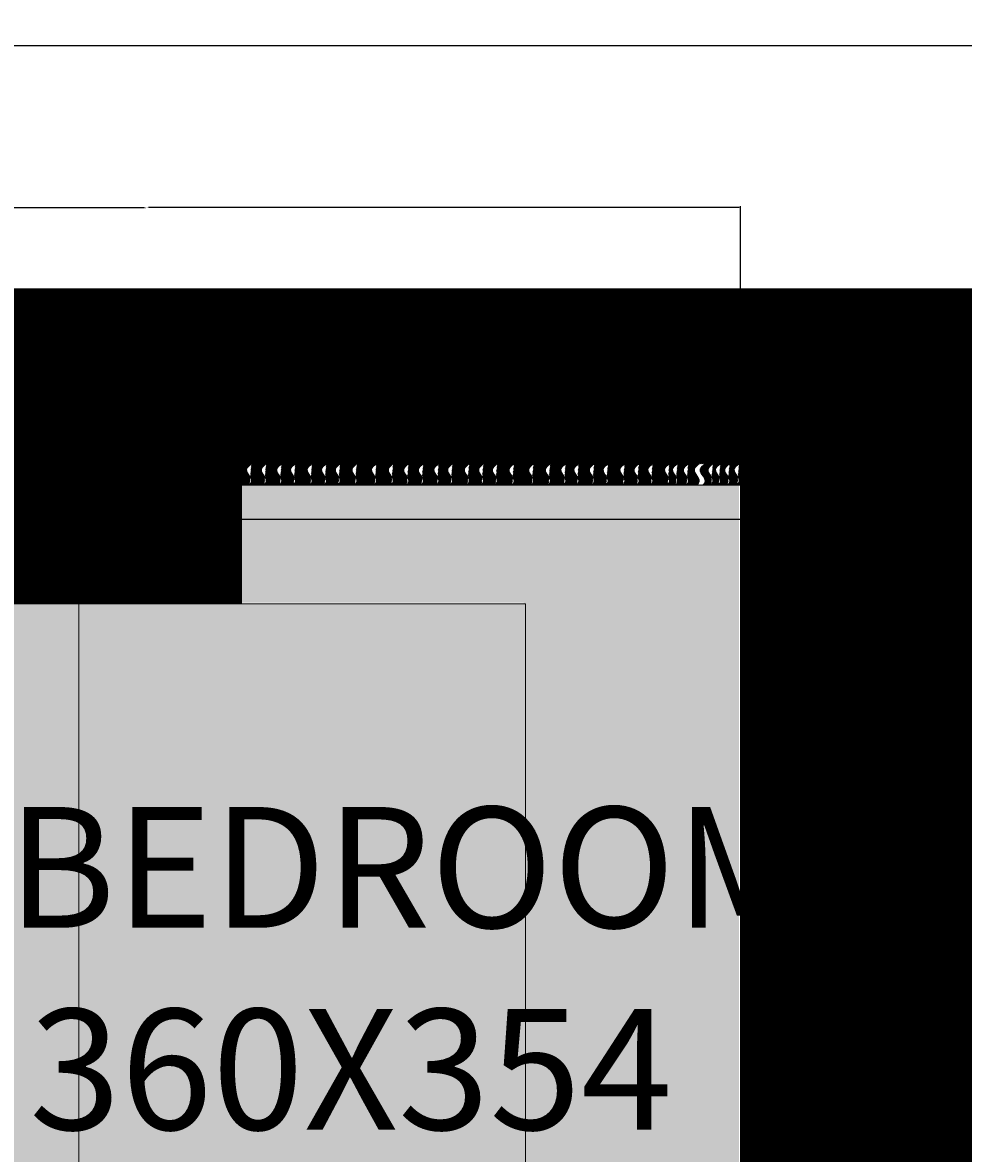
# Model space of a CAD drawing. Units: inches. Extents: x 192 to 1361, y -1362 to 367.
# Tile 8 of 23: x 361 to 495, y -616 to -454. Entities that reach past the tile are written whole.
import ezdxf

# ---------------------------------------------------------------- set-up
doc = ezdxf.new("R2010")
doc.units = ezdxf.units.IN
doc.header["$MEASUREMENT"] = 0
for name, color, linetype, lineweight in [('A-ANNO-DIMS', 2, 'Continuous', 18), ('A-AREA-IDEN', 7, 'Continuous', 18), ('A-FLOR', 8, 'Continuous', 18), ('furniture', 32, 'Continuous', 18)]:
    doc.layers.add(name, color=color, linetype=linetype, lineweight=lineweight)
doc.layers.add('A-FLOR-PATT', color=254, linetype='Continuous', lineweight=13, true_color=0xfeeab9)
doc.layers.add('A-FURN-PATT', color=254, linetype='Continuous', lineweight=13, true_color=0xfeeab9)
doc.styles.get("Standard").update_dxf_attribs({"font": 'arial.ttf'})
doc.dimstyles.get("Standard").update_dxf_attribs({"dimtxt": 0.18, "dimasz": 0.18, "dimexe": 0.18, "dimexo": 0.0625, "dimgap": 0.09, "dimtad": 0, "dimtih": 1, "dimtoh": 1, "dimzin": 0, "dimdsep": 46, "dimlunit": 3, "dimtxsty": 'Standard', "dimcen": 0.09, "dimadec": 0, "dimazin": 0, "dimtfac": 1, "dimtofl": 0, "dimtmove": 0, "dimatfit": 3, "dimfxl": 1, "dimtolj": 1, "dimtzin": 0, "dimarcsym": 0})

# ---------------------------------------------------------------- blocks, each defined once
blk = doc.blocks.new('CARPET')
at = {"layer": 'furniture'}
for p, q in [((-51.535, -98.109), (-51.535, -55.124)), ((-51.535, -55.124), (-41.267, -55.124)), ((51.553, -98.109), (-51.535, -98.109))]:
    blk.add_line(p, q, dxfattribs=at)
for points, knots in [([(-53.374, -55.995), (-53.215, -55.797), (-52.902, -55.407), (-52.343, -55.797), (-51.889, -56.079), (-51.645, -55.906), (-51.535, -55.827)], [0, 0, 0, 0, 0.653278, 1.290138, 1.740457, 2.114451, 2.114451, 2.114451, 2.114451]), ([(-53.374, -57.263), (-53.215, -57.065), (-52.902, -56.675), (-52.343, -57.065), (-51.889, -57.347), (-51.645, -57.174), (-51.535, -57.095)], [0, 0, 0, 0, 0.653278, 1.290138, 1.740457, 2.114451, 2.114451, 2.114451, 2.114451]), ([(-53.374, -58.593), (-53.215, -58.395), (-52.902, -58.005), (-52.343, -58.395), (-51.889, -58.678), (-51.645, -58.504), (-51.535, -58.426)], [0, 0, 0, 0, 0.653278, 1.290138, 1.740457, 2.114451, 2.114451, 2.114451, 2.114451]), ([(-53.374, -59.78), (-53.215, -59.582), (-52.902, -59.192), (-52.343, -59.582), (-51.889, -59.864), (-51.645, -59.691), (-51.535, -59.612)], [0, 0, 0, 0, 0.653278, 1.290138, 1.740457, 2.114451, 2.114451, 2.114451, 2.114451]), ([(-53.374, -61.218), (-53.215, -61.02), (-52.902, -60.63), (-52.343, -61.02), (-51.889, -61.302), (-51.645, -61.129), (-51.535, -61.051)], [0, 0, 0, 0, 0.653278, 1.290138, 1.740457, 2.114451, 2.114451, 2.114451, 2.114451]), ([(-53.374, -62.444), (-53.215, -62.247), (-52.902, -61.857), (-52.343, -62.247), (-51.889, -62.529), (-51.645, -62.355), (-51.535, -62.277)], [0, 0, 0, 0, 0.653278, 1.290138, 1.740457, 2.114451, 2.114451, 2.114451, 2.114451]), ([(-53.374, -63.631), (-53.215, -63.433), (-52.902, -63.043), (-52.343, -63.433), (-51.889, -63.715), (-51.645, -63.542), (-51.535, -63.463)], [0, 0, 0, 0, 0.653278, 1.290138, 1.740457, 2.114451, 2.114451, 2.114451, 2.114451]), ([(-53.374, -65.069), (-53.215, -64.872), (-52.902, -64.481), (-52.343, -64.871), (-51.889, -65.154), (-51.645, -64.98), (-51.535, -64.902)], [0, 0, 0, 0, 0.653278, 1.290138, 1.740457, 2.114451, 2.114451, 2.114451, 2.114451]), ([(-53.374, -66.759), (-53.215, -66.561), (-52.902, -66.171), (-52.343, -66.561), (-51.889, -66.844), (-51.645, -66.67), (-51.535, -66.592)], [0, 0, 0, 0, 0.653278, 1.290138, 1.740457, 2.114451, 2.114451, 2.114451, 2.114451]), ([(-53.374, -68.197), (-53.215, -68), (-52.902, -67.61), (-52.343, -68), (-51.889, -68.282), (-51.645, -68.109), (-51.535, -68.03)], [0, 0, 0, 0, 0.653278, 1.290138, 1.740457, 2.114451, 2.114451, 2.114451, 2.114451]), ([(-53.374, -69.528), (-53.215, -69.33), (-52.902, -68.94), (-52.343, -69.33), (-51.889, -69.612), (-51.645, -69.439), (-51.535, -69.36)], [0, 0, 0, 0, 0.653278, 1.290138, 1.740457, 2.114451, 2.114451, 2.114451, 2.114451]), ([(-53.374, -70.794), (-53.215, -70.596), (-52.902, -70.206), (-52.343, -70.596), (-51.889, -70.878), (-51.645, -70.705), (-51.535, -70.626)], [0, 0, 0, 0, 0.653278, 1.290138, 1.740457, 2.114451, 2.114451, 2.114451, 2.114451]), ([(-53.374, -72.124), (-53.215, -71.927), (-52.902, -71.536), (-52.343, -71.927), (-51.889, -72.209), (-51.645, -72.035), (-51.535, -71.957)], [0, 0, 0, 0, 0.653278, 1.290138, 1.740457, 2.114451, 2.114451, 2.114451, 2.114451]), ([(-53.374, -73.311), (-53.215, -73.113), (-52.902, -72.723), (-52.343, -73.113), (-51.889, -73.395), (-51.645, -73.222), (-51.535, -73.143)], [0, 0, 0, 0, 0.653278, 1.290138, 1.740457, 2.114451, 2.114451, 2.114451, 2.114451]), ([(-53.374, -74.749), (-53.215, -74.551), (-52.902, -74.161), (-52.343, -74.551), (-51.889, -74.833), (-51.645, -74.66), (-51.535, -74.582)], [0, 0, 0, 0, 0.653278, 1.290138, 1.740457, 2.114451, 2.114451, 2.114451, 2.114451]), ([(-53.374, -75.975), (-53.215, -75.778), (-52.902, -75.388), (-52.343, -75.778), (-51.889, -76.06), (-51.645, -75.887), (-51.535, -75.808)], [0, 0, 0, 0, 0.653278, 1.290138, 1.740457, 2.114451, 2.114451, 2.114451, 2.114451]), ([(-53.374, -77.162), (-53.215, -76.964), (-52.902, -76.574), (-52.343, -76.964), (-51.889, -77.246), (-51.645, -77.073), (-51.535, -76.995)], [0, 0, 0, 0, 0.653278, 1.290138, 1.740457, 2.114451, 2.114451, 2.114451, 2.114451]), ([(-53.374, -78.6), (-53.215, -78.403), (-52.902, -78.012), (-52.343, -78.403), (-51.889, -78.685), (-51.645, -78.511), (-51.535, -78.433)], [0, 0, 0, 0, 0.653278, 1.290138, 1.740457, 2.114451, 2.114451, 2.114451, 2.114451]), ([(-53.374, -80.29), (-53.215, -80.093), (-52.902, -79.702), (-52.343, -80.093), (-51.889, -80.375), (-51.645, -80.201), (-51.535, -80.123)], [0, 0, 0, 0, 0.653278, 1.290138, 1.740457, 2.114451, 2.114451, 2.114451, 2.114451]), ([(-53.374, -81.728), (-53.215, -81.531), (-52.902, -81.141), (-52.343, -81.531), (-51.889, -81.813), (-51.645, -81.64), (-51.535, -81.561)], [0, 0, 0, 0, 0.653278, 1.290138, 1.740457, 2.114451, 2.114451, 2.114451, 2.114451]), ([(-53.374, -83.059), (-53.215, -82.861), (-52.902, -82.471), (-52.343, -82.861), (-51.889, -83.143), (-51.645, -82.97), (-51.535, -82.891)], [0, 0, 0, 0, 0.653278, 1.290138, 1.740457, 2.114451, 2.114451, 2.114451, 2.114451]), ([(-53.374, -84.183), (-53.215, -83.985), (-52.902, -83.595), (-52.343, -83.985), (-51.889, -84.267), (-51.645, -84.094), (-51.535, -84.015)], [0, 0, 0, 0, 0.653278, 1.290138, 1.740457, 2.114451, 2.114451, 2.114451, 2.114451]), ([(-53.374, -85.513), (-53.215, -85.316), (-52.902, -84.926), (-52.343, -85.316), (-51.889, -85.598), (-51.645, -85.424), (-51.535, -85.346)], [0, 0, 0, 0, 0.653278, 1.290138, 1.740457, 2.114451, 2.114451, 2.114451, 2.114451]), ([(-53.374, -86.7), (-53.215, -86.502), (-52.902, -86.112), (-52.343, -86.502), (-51.889, -86.784), (-51.645, -86.611), (-51.535, -86.532)], [0, 0, 0, 0, 0.653278, 1.290138, 1.740457, 2.114451, 2.114451, 2.114451, 2.114451]), ([(-53.374, -88.138), (-53.215, -87.941), (-52.902, -87.55), (-52.343, -87.94), (-51.889, -88.223), (-51.645, -88.049), (-51.535, -87.971)], [0, 0, 0, 0, 0.653278, 1.290138, 1.740457, 2.114451, 2.114451, 2.114451, 2.114451]), ([(-53.374, -89.364), (-53.215, -89.167), (-52.902, -88.777), (-52.343, -89.167), (-51.889, -89.449), (-51.645, -89.276), (-51.535, -89.197)], [0, 0, 0, 0, 0.653278, 1.290138, 1.740457, 2.114451, 2.114451, 2.114451, 2.114451]), ([(-53.374, -90.551), (-53.215, -90.353), (-52.902, -89.963), (-52.343, -90.353), (-51.889, -90.635), (-51.645, -90.462), (-51.535, -90.384)], [0, 0, 0, 0, 0.653278, 1.290138, 1.740457, 2.114451, 2.114451, 2.114451, 2.114451]), ([(-53.374, -91.989), (-53.215, -91.792), (-52.902, -91.402), (-52.343, -91.792), (-51.889, -92.074), (-51.645, -91.9), (-51.535, -91.822)], [0, 0, 0, 0, 0.653278, 1.290138, 1.740457, 2.114451, 2.114451, 2.114451, 2.114451]), ([(-53.374, -92.689), (-53.216, -92.483), (-52.904, -92.076), (-52.346, -92.494), (-51.889, -92.773), (-51.645, -92.6), (-51.535, -92.522)], [0, 0, 0, 0, 0.663904, 1.307406, 1.757725, 2.131719, 2.131719, 2.131719, 2.131719]), ([(-53.374, -93.614), (-53.215, -93.416), (-52.902, -93.026), (-52.343, -93.416), (-51.889, -93.698), (-51.645, -93.525), (-51.535, -93.446)], [0, 0, 0, 0, 0.653278, 1.290138, 1.740457, 2.114451, 2.114451, 2.114451, 2.114451]), ([(-53.374, -94.548), (-53.215, -94.351), (-52.902, -93.96), (-52.343, -94.35), (-51.889, -94.633), (-51.645, -94.459), (-51.535, -94.381)], [0, 0, 0, 0, 0.653278, 1.290138, 1.740457, 2.114451, 2.114451, 2.114451, 2.114451]), ([(-53.374, -95.052), (-53.215, -94.854), (-52.902, -94.464), (-52.343, -94.854), (-51.889, -95.136), (-51.645, -94.963), (-51.535, -94.885)], [0, 0, 0, 0, 0.653278, 1.290138, 1.740457, 2.114451, 2.114451, 2.114451, 2.114451]), ([(-53.374, -95.735), (-53.215, -95.537), (-52.902, -95.147), (-52.343, -95.537), (-51.889, -95.819), (-51.645, -95.646), (-51.535, -95.567)], [0, 0, 0, 0, 0.653278, 1.290138, 1.740457, 2.114451, 2.114451, 2.114451, 2.114451]), ([(-53.374, -96.382), (-53.215, -96.185), (-52.902, -95.795), (-52.343, -96.185), (-51.889, -96.467), (-51.645, -96.294), (-51.535, -96.215)], [0, 0, 0, 0, 0.653278, 1.290138, 1.740457, 2.114451, 2.114451, 2.114451, 2.114451]), ([(-53.374, -97.173), (-53.215, -96.975), (-52.902, -96.585), (-52.343, -96.975), (-51.889, -97.257), (-51.645, -97.084), (-51.535, -97.006)], [0, 0, 0, 0, 0.653278, 1.290138, 1.740457, 2.114451, 2.114451, 2.114451, 2.114451]), ([(-53.374, -97.991), (-53.215, -97.793), (-52.902, -97.403), (-52.343, -97.793), (-51.889, -98.075), (-51.645, -97.902), (-51.535, -97.824)], [0, 0, 0, 0, 0.653278, 1.290138, 1.740457, 2.114451, 2.114451, 2.114451, 2.114451])]:
    blk.add_open_spline(points, degree=3, knots=knots, dxfattribs=at)
blk = doc.blocks.new('A$C58D270C6')
at = {"layer": 'furniture'}
blk.add_line((42.078, 108), (42.078, 36), dxfattribs=at)
blk.add_lwpolyline([(0, 108), (77.905, 108), (77.905, 36), (0, 36)], close=True, dxfattribs=at)
at = {"layer": 'furniture', "xscale": 0.9312884925094044, "yscale": 0.9312884925094044, "zscale": 0.9312884925094044, "rotation": 90}
blk.add_blockref('CARPET', (3.79, 74.474), dxfattribs=at)
blk = doc.blocks.new('*D23')
at = {"layer": 'A-ANNO-DIMS', "color": 0, "lineweight": -2, "transparency": 16777216}
for p, q in [((463.14, -508.44), (491.09, -508.44)), ((490.91, -508.62), (490.91, -601.06)), ((490.91, -693.87), (490.91, -601.42)), ((463.14, -694.05), (491.09, -694.05))]:
    blk.add_line(p, q, dxfattribs=at)
at = {"layer": 'A-ANNO-DIMS', "color": 0, "transparency": 16777216}
for points in [[(490.88, -508.62), (490.94, -508.62), (490.91, -508.44)], [(490.88, -693.87), (490.94, -693.87), (490.91, -694.05)]]:
    blk.add_solid(points, dxfattribs=at)
at = {"layer": 'Defpoints', "color": 0, "transparency": 16777216}
for p in [(463.07, -508.44), (463.07, -694.05), (490.91, -694.05)]:
    blk.add_point(p, dxfattribs=at)
at = {"layer": 'A-ANNO-DIMS', "color": 0, "transparency": 16777216, "insert": (490.91, -601.24), "char_height": 0.18, "attachment_point": 5}
blk.add_mtext('\\A1;BED 186', dxfattribs=at)
blk = doc.blocks.new('*D24')
at = {"layer": 'A-ANNO-DIMS', "color": 0, "lineweight": -2, "transparency": 16777216}
for p, q in [((293.48, -508.38), (293.48, -480.42)), ((293.66, -480.6), (378, -480.6)), ((462.89, -480.6), (378.56, -480.6)), ((463.07, -508.38), (463.07, -480.42))]:
    blk.add_line(p, q, dxfattribs=at)
at = {"layer": 'A-ANNO-DIMS', "color": 0, "transparency": 16777216}
for points in [[(293.66, -480.57), (293.66, -480.63), (293.48, -480.6)], [(462.89, -480.57), (462.89, -480.63), (463.07, -480.6)]]:
    blk.add_solid(points, dxfattribs=at)
at = {"layer": 'Defpoints', "color": 0, "transparency": 16777216}
for p in [(463.07, -480.6), (293.48, -508.44), (463.07, -508.44)]:
    blk.add_point(p, dxfattribs=at)
at = {"layer": 'A-ANNO-DIMS', "color": 0, "transparency": 16777216, "insert": (378.28, -480.6), "char_height": 0.18, "attachment_point": 5}
blk.add_mtext('\\A1;170', dxfattribs=at)
blk = doc.blocks.new('*D48')
at = {"layer": 'A-ANNO-DIMS', "color": 0, "lineweight": -2, "transparency": 16777216}
for p, q in [((325.63, 258.53), (192.16, 258.53)), ((192.34, 258.35), (192.34, -429.22)), ((192.34, -1117.14), (192.34, -429.58)), ((395.21, -1117.32), (192.16, -1117.32))]:
    blk.add_line(p, q, dxfattribs=at)
at = {"layer": 'A-ANNO-DIMS', "color": 0, "transparency": 16777216}
for points in [[(192.31, 258.35), (192.37, 258.35), (192.34, 258.53)], [(192.31, -1117.14), (192.37, -1117.14), (192.34, -1117.32)]]:
    blk.add_solid(points, dxfattribs=at)
at = {"layer": 'Defpoints', "color": 0, "transparency": 16777216}
for p in [(325.7, 258.53), (192.34, -1117.32), (395.28, -1117.32)]:
    blk.add_point(p, dxfattribs=at)
at = {"layer": 'A-ANNO-DIMS', "color": 0, "transparency": 16777216, "insert": (192.34, -429.4), "char_height": 0.18, "attachment_point": 5}
blk.add_mtext('\\A1;1375.9', dxfattribs=at)
blk = doc.blocks.new('*D69')
at = {"layer": 'A-ANNO-DIMS', "color": 0, "lineweight": -2, "transparency": 16777216}
for p, q in [((981.75, -457.5), (192.16, -457.5)), ((192.34, -457.68), (192.34, -491.13)), ((192.34, -524.95), (192.34, -491.5)), ((980.52, -525.13), (192.16, -525.13))]:
    blk.add_line(p, q, dxfattribs=at)
at = {"layer": 'A-ANNO-DIMS', "color": 0, "transparency": 16777216}
for points in [[(192.31, -457.68), (192.37, -457.68), (192.34, -457.5)], [(192.31, -524.95), (192.37, -524.95), (192.34, -525.13)]]:
    blk.add_solid(points, dxfattribs=at)
at = {"layer": 'Defpoints', "color": 0, "transparency": 16777216}
for p in [(981.81, -457.5), (192.34, -525.13), (980.58, -525.13)]:
    blk.add_point(p, dxfattribs=at)
at = {"layer": 'A-ANNO-DIMS', "color": 0, "transparency": 16777216, "insert": (192.34, -491.31), "char_height": 0.18, "attachment_point": 5}
blk.add_mtext('\\A1;67.63', dxfattribs=at)

msp = doc.modelspace()

# ---------------------------------------------------------------- hatches: boundary and pattern name
at = {"layer": 'A-FLOR-PATT'}
h = msp.add_hatch(dxfattribs=at)
h.set_pattern_fill('ANSI31', color=256)
edge = h.paths.add_edge_path()
edge.add_line((513.1511, -492.1899), (327.1032, -492.1899))
edge.add_line((327.1032, -492.1899), (327.1032, -508.439))
edge.add_line((327.1032, -508.439), (326.9465, -508.439))
edge.add_line((326.9465, -508.439), (326.6697, -537.1419))
edge.add_line((326.6697, -537.1419), (391.8439, -537.1419))
edge.add_line((391.8439, -537.1419), (391.8439, -520.2026))
edge.add_line((391.8439, -520.2026), (393.0084, -520.2026))
edge.add_spline(control_points=[(393.2858, -517.1545), (392.9584, -517.4172), (392.3119, -517.936), (392.9583, -518.8629), (393.4257, -519.6151), (393.1386, -520.0192), (393.0084, -520.2026)], knot_values=[0, 0, 0, 0, 0.65327829, 1.2901376, 1.74045698, 2.11445126, 2.11445126, 2.11445126, 2.11445126], degree=3, periodic=0)
edge.add_line((393.0084, -520.2026), (395.1098, -520.2026))
edge.add_spline(control_points=[(395.3872, -517.1545), (395.0598, -517.4172), (394.4133, -517.936), (395.0598, -518.8629), (395.5272, -519.6151), (395.2401, -520.0192), (395.1098, -520.2026)], knot_values=[0, 0, 0, 0, 0.65327829, 1.2901376, 1.74045698, 2.11445126, 2.11445126, 2.11445126, 2.11445126], degree=3, periodic=0)
edge.add_line((395.1098, -520.2026), (397.3144, -520.2026))
edge.add_spline(control_points=[(397.5918, -517.1545), (397.2644, -517.4172), (396.6179, -517.936), (397.2643, -518.8629), (397.7317, -519.6151), (397.4446, -520.0192), (397.3144, -520.2026)], knot_values=[0, 0, 0, 0, 0.65327829, 1.2901376, 1.74045698, 2.11445126, 2.11445126, 2.11445126, 2.11445126], degree=3, periodic=0)
edge.add_line((397.3144, -520.2026), (399.2806, -520.2026))
edge.add_spline(control_points=[(399.558, -517.1545), (399.2307, -517.4172), (398.5841, -517.936), (399.2306, -518.8629), (399.698, -519.6151), (399.4109, -520.0192), (399.2806, -520.2026)], knot_values=[0, 0, 0, 0, 0.65327829, 1.2901376, 1.74045698, 2.11445126, 2.11445126, 2.11445126, 2.11445126], degree=3, periodic=0)
edge.add_line((399.2806, -520.2026), (401.664, -520.2026))
edge.add_spline(control_points=[(401.9414, -517.1545), (401.614, -517.4172), (400.9675, -517.936), (401.6139, -518.8629), (402.0814, -519.6151), (401.7943, -520.0192), (401.664, -520.2026)], knot_values=[0, 0, 0, 0, 0.65327829, 1.2901376, 1.74045698, 2.11445126, 2.11445126, 2.11445126, 2.11445126], degree=3, periodic=0)
edge.add_line((401.664, -520.2026), (403.6961, -520.2026))
edge.add_spline(control_points=[(403.9735, -517.1545), (403.6461, -517.4172), (402.9996, -517.936), (403.6461, -518.8629), (404.1135, -519.6151), (403.8264, -520.0192), (403.6961, -520.2026)], knot_values=[0, 0, 0, 0, 0.65327829, 1.2901376, 1.74045698, 2.11445126, 2.11445126, 2.11445126, 2.11445126], degree=3, periodic=0)
edge.add_line((403.6961, -520.2026), (405.6624, -520.2026))
edge.add_spline(control_points=[(405.9398, -517.1545), (405.6124, -517.4172), (404.9659, -517.936), (405.6123, -518.8629), (406.0797, -519.6151), (405.7926, -520.0192), (405.6624, -520.2026)], knot_values=[0, 0, 0, 0, 0.65327829, 1.2901376, 1.74045698, 2.11445126, 2.11445126, 2.11445126, 2.11445126], degree=3, periodic=0)
edge.add_line((405.6624, -520.2026), (408.0457, -520.2026))
edge.add_spline(control_points=[(408.3231, -517.1545), (407.9958, -517.4172), (407.3493, -517.936), (407.9957, -518.8629), (408.4631, -519.6151), (408.176, -520.0192), (408.0457, -520.2026)], knot_values=[0, 0, 0, 0, 0.65327829, 1.2901376, 1.74045698, 2.11445126, 2.11445126, 2.11445126, 2.11445126], degree=3, periodic=0)
edge.add_line((408.0457, -520.2026), (410.8462, -520.2026))
edge.add_spline(control_points=[(411.1236, -517.1545), (410.7962, -517.4172), (410.1497, -517.936), (410.7961, -518.8629), (411.2635, -519.6151), (410.9764, -520.0192), (410.8462, -520.2026)], knot_values=[0, 0, 0, 0, 0.65327829, 1.2901376, 1.74045698, 2.11445126, 2.11445126, 2.11445126, 2.11445126], degree=3, periodic=0)
edge.add_line((410.8462, -520.2026), (413.2295, -520.2026))
edge.add_spline(control_points=[(413.5069, -517.1545), (413.1795, -517.4172), (412.533, -517.936), (413.1794, -518.8629), (413.6468, -519.6151), (413.3597, -520.0192), (413.2295, -520.2026)], knot_values=[0, 0, 0, 0, 0.65327829, 1.2901376, 1.74045698, 2.11445126, 2.11445126, 2.11445126, 2.11445126], degree=3, periodic=0)
edge.add_line((413.2295, -520.2026), (415.434, -520.2026))
edge.add_spline(control_points=[(415.7114, -517.1545), (415.3841, -517.4172), (414.7376, -517.936), (415.384, -518.8629), (415.8514, -519.6151), (415.5643, -520.0192), (415.434, -520.2026)], knot_values=[0, 0, 0, 0, 0.65327829, 1.2901376, 1.74045698, 2.11445126, 2.11445126, 2.11445126, 2.11445126], degree=3, periodic=0)
edge.add_line((415.434, -520.2026), (417.5321, -520.2026))
edge.add_spline(control_points=[(417.8095, -517.1545), (417.4821, -517.4172), (416.8356, -517.936), (417.482, -518.8629), (417.9494, -519.6151), (417.6623, -520.0192), (417.5321, -520.2026)], knot_values=[0, 0, 0, 0, 0.65327829, 1.2901376, 1.74045698, 2.11445126, 2.11445126, 2.11445126, 2.11445126], degree=3, periodic=0)
edge.add_line((417.5321, -520.2026), (419.7366, -520.2026))
edge.add_spline(control_points=[(420.014, -517.1545), (419.6867, -517.4172), (419.0401, -517.936), (419.6866, -518.8629), (420.154, -519.6151), (419.8669, -520.0192), (419.7366, -520.2026)], knot_values=[0, 0, 0, 0, 0.65327829, 1.2901376, 1.74045698, 2.11445126, 2.11445126, 2.11445126, 2.11445126], degree=3, periodic=0)
edge.add_line((419.7366, -520.2026), (421.7029, -520.2026))
edge.add_spline(control_points=[(421.9803, -517.1545), (421.6529, -517.4172), (421.0064, -517.936), (421.6528, -518.8629), (422.1202, -519.6151), (421.8331, -520.0192), (421.7029, -520.2026)], knot_values=[0, 0, 0, 0, 0.65327829, 1.2901376, 1.74045698, 2.11445126, 2.11445126, 2.11445126, 2.11445126], degree=3, periodic=0)
edge.add_line((421.7029, -520.2026), (424.0863, -520.2026))
edge.add_spline(control_points=[(424.3637, -517.1545), (424.0363, -517.4172), (423.3898, -517.936), (424.0362, -518.8629), (424.5036, -519.6151), (424.2165, -520.0192), (424.0863, -520.2026)], knot_values=[0, 0, 0, 0, 0.65327829, 1.2901376, 1.74045698, 2.11445126, 2.11445126, 2.11445126, 2.11445126], degree=3, periodic=0)
edge.add_line((424.0863, -520.2026), (426.1184, -520.2026))
edge.add_spline(control_points=[(426.3958, -517.1545), (426.0684, -517.4172), (425.4219, -517.936), (426.0683, -518.8629), (426.5357, -519.6151), (426.2486, -520.0192), (426.1184, -520.2026)], knot_values=[0, 0, 0, 0, 0.65327829, 1.2901376, 1.74045698, 2.11445126, 2.11445126, 2.11445126, 2.11445126], degree=3, periodic=0)
edge.add_line((426.1184, -520.2026), (428.0846, -520.2026))
edge.add_spline(control_points=[(428.362, -517.1545), (428.0346, -517.4172), (427.3881, -517.936), (428.0346, -518.8629), (428.502, -519.6151), (428.2149, -520.0192), (428.0846, -520.2026)], knot_values=[0, 0, 0, 0, 0.65327829, 1.2901376, 1.74045698, 2.11445126, 2.11445126, 2.11445126, 2.11445126], degree=3, periodic=0)
edge.add_line((428.0846, -520.2026), (430.468, -520.2026))
edge.add_spline(control_points=[(430.7454, -517.1545), (430.418, -517.4172), (429.7715, -517.936), (430.4179, -518.8629), (430.8853, -519.6151), (430.5983, -520.0192), (430.468, -520.2026)], knot_values=[0, 0, 0, 0, 0.65327829, 1.2901376, 1.74045698, 2.11445126, 2.11445126, 2.11445126, 2.11445126], degree=3, periodic=0)
edge.add_line((430.468, -520.2026), (433.2684, -520.2026))
edge.add_spline(control_points=[(433.5458, -517.1545), (433.2184, -517.4172), (432.5719, -517.936), (433.2184, -518.8629), (433.6858, -519.6151), (433.3987, -520.0192), (433.2684, -520.2026)], knot_values=[0, 0, 0, 0, 0.65327829, 1.2901376, 1.74045698, 2.11445126, 2.11445126, 2.11445126, 2.11445126], degree=3, periodic=0)
edge.add_line((433.2684, -520.2026), (435.6517, -520.2026))
edge.add_spline(control_points=[(435.9291, -517.1545), (435.6017, -517.4172), (434.9552, -517.936), (435.6017, -518.8629), (436.0691, -519.6151), (435.782, -520.0192), (435.6517, -520.2026)], knot_values=[0, 0, 0, 0, 0.65327829, 1.2901376, 1.74045698, 2.11445126, 2.11445126, 2.11445126, 2.11445126], degree=3, periodic=0)
edge.add_line((435.6517, -520.2026), (437.8563, -520.2026))
edge.add_spline(control_points=[(438.1337, -517.1545), (437.8063, -517.4172), (437.1598, -517.936), (437.8062, -518.8629), (438.2736, -519.6151), (437.9865, -520.0192), (437.8563, -520.2026)], knot_values=[0, 0, 0, 0, 0.65327829, 1.2901376, 1.74045698, 2.11445126, 2.11445126, 2.11445126, 2.11445126], degree=3, periodic=0)
edge.add_line((437.8563, -520.2026), (439.7189, -520.2026))
edge.add_spline(control_points=[(439.9963, -517.1545), (439.669, -517.4172), (439.0225, -517.936), (439.6689, -518.8629), (440.1363, -519.6151), (439.8492, -520.0192), (439.7189, -520.2026)], knot_values=[0, 0, 0, 0, 0.65327829, 1.2901376, 1.74045698, 2.11445126, 2.11445126, 2.11445126, 2.11445126], degree=3, periodic=0)
edge.add_line((439.7189, -520.2026), (441.9235, -520.2026))
edge.add_spline(control_points=[(442.2009, -517.1545), (441.8735, -517.4172), (441.227, -517.936), (441.8735, -518.8629), (442.3409, -519.6151), (442.0538, -520.0192), (441.9235, -520.2026)], knot_values=[0, 0, 0, 0, 0.65327829, 1.2901376, 1.74045698, 2.11445126, 2.11445126, 2.11445126, 2.11445126], degree=3, periodic=0)
edge.add_line((441.9235, -520.2026), (443.8898, -520.2026))
edge.add_spline(control_points=[(444.1672, -517.1545), (443.8398, -517.4172), (443.1933, -517.936), (443.8397, -518.8629), (444.3071, -519.6151), (444.02, -520.0192), (443.8898, -520.2026)], knot_values=[0, 0, 0, 0, 0.65327829, 1.2901376, 1.74045698, 2.11445126, 2.11445126, 2.11445126, 2.11445126], degree=3, periodic=0)
edge.add_line((443.8898, -520.2026), (446.2731, -520.2026))
edge.add_spline(control_points=[(446.5505, -517.1545), (446.2232, -517.4172), (445.5767, -517.936), (446.2231, -518.8629), (446.6905, -519.6151), (446.4034, -520.0192), (446.2731, -520.2026)], knot_values=[0, 0, 0, 0, 0.65327829, 1.2901376, 1.74045698, 2.11445126, 2.11445126, 2.11445126, 2.11445126], degree=3, periodic=0)
edge.add_line((446.2731, -520.2026), (448.3052, -520.2026))
edge.add_spline(control_points=[(448.5826, -517.1545), (448.2553, -517.4172), (447.6088, -517.936), (448.2552, -518.8629), (448.7226, -519.6151), (448.4355, -520.0192), (448.3052, -520.2026)], knot_values=[0, 0, 0, 0, 0.65327829, 1.2901376, 1.74045698, 2.11445126, 2.11445126, 2.11445126, 2.11445126], degree=3, periodic=0)
edge.add_line((448.3052, -520.2026), (450.2715, -520.2026))
edge.add_spline(control_points=[(450.5489, -517.1545), (450.2215, -517.4172), (449.575, -517.936), (450.2214, -518.8629), (450.6888, -519.6151), (450.4018, -520.0192), (450.2715, -520.2026)], knot_values=[0, 0, 0, 0, 0.65327829, 1.2901376, 1.74045698, 2.11445126, 2.11445126, 2.11445126, 2.11445126], degree=3, periodic=0)
edge.add_line((450.2715, -520.2026), (452.6549, -520.2026))
edge.add_spline(control_points=[(452.9323, -517.1545), (452.6049, -517.4172), (451.9584, -517.936), (452.6048, -518.8629), (453.0722, -519.6151), (452.7851, -520.0192), (452.6549, -520.2026)], knot_values=[0, 0, 0, 0, 0.65327829, 1.2901376, 1.74045698, 2.11445126, 2.11445126, 2.11445126, 2.11445126], degree=3, periodic=0)
edge.add_line((452.6549, -520.2026), (453.8151, -520.2026))
edge.add_spline(control_points=[(454.0925, -517.1545), (453.7499, -517.417), (453.0754, -517.9338), (453.769, -518.8576), (454.2314, -519.6154), (453.945, -520.0193), (453.8151, -520.2026)], knot_values=[0, 0, 0, 0, 0.6639037, 1.30740562, 1.757725, 2.13171928, 2.13171928, 2.13171928, 2.13171928], degree=3, periodic=0)
edge.add_line((453.8151, -520.2026), (455.3467, -520.2026))
edge.add_spline(control_points=[(455.6241, -517.1545), (455.2967, -517.4172), (454.6502, -517.936), (455.2967, -518.8629), (455.7641, -519.6151), (455.477, -520.0192), (455.3467, -520.2026)], knot_values=[0, 0, 0, 0, 0.65327829, 1.2901376, 1.74045698, 2.11445126, 2.11445126, 2.11445126, 2.11445126], degree=3, periodic=0)
edge.add_line((455.3467, -520.2026), (456.895, -520.2026))
edge.add_spline(control_points=[(456.895, -520.2026), (457.0253, -520.0192), (457.3124, -519.6151), (456.845, -518.8629), (456.1986, -517.936), (456.8451, -517.4172), (457.1724, -517.1545)], knot_values=[0, 0, 0, 0, 0.37399428, 0.82431366, 1.46117297, 2.11445126, 2.11445126, 2.11445126, 2.11445126], degree=3, periodic=0)
edge.add_spline(control_points=[(458.0074, -517.1545), (457.68, -517.4172), (457.0335, -517.936), (457.68, -518.8629), (458.1474, -519.6151), (457.8603, -520.0192), (457.73, -520.2026)], knot_values=[0, 0, 0, 0, 0.65327829, 1.2901376, 1.74045698, 2.11445126, 2.11445126, 2.11445126, 2.11445126], degree=3, periodic=0)
edge.add_line((457.73, -520.2026), (458.8613, -520.2026))
edge.add_spline(control_points=[(459.1387, -517.1545), (458.8113, -517.4172), (458.1648, -517.936), (458.8112, -518.8629), (459.2786, -519.6151), (458.9916, -520.0192), (458.8613, -520.2026)], knot_values=[0, 0, 0, 0, 0.65327829, 1.2901376, 1.74045698, 2.11445126, 2.11445126, 2.11445126, 2.11445126], degree=3, periodic=0)
edge.add_line((458.8613, -520.2026), (459.9346, -520.2026))
edge.add_spline(control_points=[(460.212, -517.1545), (459.8846, -517.4172), (459.2381, -517.936), (459.8845, -518.8629), (460.3519, -519.6151), (460.0648, -520.0192), (459.9346, -520.2026)], knot_values=[0, 0, 0, 0, 0.65327829, 1.2901376, 1.74045698, 2.11445126, 2.11445126, 2.11445126, 2.11445126], degree=3, periodic=0)
edge.add_line((459.9346, -520.2026), (461.2447, -520.2026))
edge.add_spline(control_points=[(461.5221, -517.1545), (461.1947, -517.4172), (460.5482, -517.936), (461.1946, -518.8629), (461.662, -519.6151), (461.3749, -520.0192), (461.2447, -520.2026)], knot_values=[0, 0, 0, 0, 0.65327829, 1.2901376, 1.74045698, 2.11445126, 2.11445126, 2.11445126, 2.11445126], degree=3, periodic=0)
edge.add_line((461.2447, -520.2026), (462.6002, -520.2026))
edge.add_spline(control_points=[(462.8776, -517.1545), (462.5502, -517.4172), (461.9037, -517.936), (462.5501, -518.8629), (463.0175, -519.6151), (462.7304, -520.0192), (462.6002, -520.2026)], knot_values=[0, 0, 0, 0, 0.65327829, 1.2901376, 1.74045698, 2.11445126, 2.11445126, 2.11445126, 2.11445126], degree=3, periodic=0)
edge.add_line((462.6002, -520.2026), (463.0739, -520.2026))
edge.add_line((463.0739, -520.2026), (463.0739, -691.0271))
edge.add_line((463.0739, -691.0271), (462.6214, -691.0271))
edge.add_spline(control_points=[(462.8776, -694.0453), (462.5502, -693.7826), (461.9037, -693.2638), (462.5501, -692.3369), (463.011, -691.5951), (462.7443, -691.2005), (462.6214, -691.0271)], knot_values=[0, 0, 0, 0, 0.65327829, 1.2901376, 1.74045698, 2.09412198, 2.09412198, 2.09412198, 2.09412198], degree=3, periodic=0)
edge.add_line((462.6214, -691.0271), (461.3416, -691.0271))
edge.add_spline(control_points=[(461.5978, -694.0453), (461.2704, -693.7826), (460.6239, -693.2638), (461.2703, -692.3369), (461.7312, -691.5951), (461.4644, -691.2005), (461.3416, -691.0271)], knot_values=[0, 0, 0, 0, 0.65327829, 1.2901376, 1.74045698, 2.09412198, 2.09412198, 2.09412198, 2.09412198], degree=3, periodic=0)
edge.add_line((461.3416, -691.0271), (460.0315, -691.0271))
edge.add_spline(control_points=[(460.2877, -694.0453), (459.9603, -693.7826), (459.3138, -693.2638), (459.9602, -692.3369), (460.4211, -691.5951), (460.1544, -691.2005), (460.0315, -691.0271)], knot_values=[0, 0, 0, 0, 0.65327829, 1.2901376, 1.74045698, 2.09412198, 2.09412198, 2.09412198, 2.09412198], degree=3, periodic=0)
edge.add_line((460.0315, -691.0271), (458.9582, -691.0271))
edge.add_spline(control_points=[(459.2144, -694.0453), (458.887, -693.7826), (458.2405, -693.2638), (458.8869, -692.3369), (459.3478, -691.5951), (459.0811, -691.2005), (458.9582, -691.0271)], knot_values=[0, 0, 0, 0, 0.65327829, 1.2901376, 1.74045698, 2.09412198, 2.09412198, 2.09412198, 2.09412198], degree=3, periodic=0)
edge.add_line((458.9582, -691.0271), (457.8269, -691.0271))
edge.add_spline(control_points=[(457.8269, -691.0271), (457.9464, -691.2008), (458.2187, -691.5966), (457.7545, -692.3366), (457.1096, -693.2638), (457.7558, -693.7826), (458.0831, -694.0453)], knot_values=[0, 0, 0, 0, 0.3521435, 0.80246288, 1.43932219, 2.09260048, 2.09260048, 2.09260048, 2.09260048], degree=3, periodic=0)
edge.add_spline(control_points=[(457.2481, -694.0453), (456.9209, -693.7826), (456.2746, -693.2638), (456.9195, -692.3366), (457.3837, -691.5966), (457.1114, -691.2008), (456.992, -691.0271)], knot_values=[0, 0, 0, 0, 0.65327829, 1.2901376, 1.74045698, 2.09260048, 2.09260048, 2.09260048, 2.09260048], degree=3, periodic=0)
edge.add_line((456.992, -691.0271), (455.4436, -691.0271))
edge.add_spline(control_points=[(455.6998, -694.0453), (455.3725, -693.7826), (454.7263, -693.2638), (455.3712, -692.3366), (455.8354, -691.5966), (455.5631, -691.2008), (455.4436, -691.0271)], knot_values=[0, 0, 0, 0, 0.65327829, 1.2901376, 1.74045698, 2.09260048, 2.09260048, 2.09260048, 2.09260048], degree=3, periodic=0)
edge.add_line((455.4436, -691.0271), (453.8363, -691.0271))
edge.add_spline(control_points=[(454.0925, -694.0453), (453.7602, -693.7827), (453.1046, -693.2646), (453.7653, -692.3383), (454.2277, -691.5965), (453.9557, -691.2008), (453.8363, -691.0271)], knot_values=[0, 0, 0, 0, 0.65679228, 1.29582582, 1.7461452, 2.0982924, 2.0982924, 2.0982924, 2.0982924], degree=3, periodic=0)
edge.add_line((453.8363, -691.0271), (452.6761, -691.0271))
edge.add_spline(control_points=[(452.9323, -694.0453), (452.605, -693.7826), (451.9587, -693.2638), (452.6037, -692.3366), (453.0678, -691.5966), (452.7956, -691.2008), (452.6761, -691.0271)], knot_values=[0, 0, 0, 0, 0.65327829, 1.2901376, 1.74045698, 2.09260048, 2.09260048, 2.09260048, 2.09260048], degree=3, periodic=0)
edge.add_line((452.6761, -691.0271), (450.2927, -691.0271))
edge.add_spline(control_points=[(450.5489, -694.0453), (450.2216, -693.7826), (449.5753, -693.2638), (450.2203, -692.3366), (450.6845, -691.5966), (450.4122, -691.2008), (450.2927, -691.0271)], knot_values=[0, 0, 0, 0, 0.65327829, 1.2901376, 1.74045698, 2.09260048, 2.09260048, 2.09260048, 2.09260048], degree=3, periodic=0)
edge.add_line((450.2927, -691.0271), (448.3265, -691.0271))
edge.add_spline(control_points=[(448.5826, -694.0453), (448.2553, -693.7826), (447.6088, -693.2638), (448.2552, -692.3369), (448.7161, -691.5951), (448.4493, -691.2005), (448.3265, -691.0271)], knot_values=[0, 0, 0, 0, 0.65327829, 1.2901376, 1.74045698, 2.09412198, 2.09412198, 2.09412198, 2.09412198], degree=3, periodic=0)
edge.add_line((448.3265, -691.0271), (446.2944, -691.0271))
edge.add_spline(control_points=[(446.5505, -694.0453), (446.2232, -693.7826), (445.5767, -693.2638), (446.2231, -692.3369), (446.684, -691.5951), (446.4172, -691.2005), (446.2944, -691.0271)], knot_values=[0, 0, 0, 0, 0.65327829, 1.2901376, 1.74045698, 2.09412198, 2.09412198, 2.09412198, 2.09412198], degree=3, periodic=0)
edge.add_line((446.2944, -691.0271), (443.911, -691.0271))
edge.add_spline(control_points=[(444.1672, -694.0453), (443.8398, -693.7826), (443.1933, -693.2638), (443.8397, -692.3369), (444.3006, -691.5951), (444.0338, -691.2005), (443.911, -691.0271)], knot_values=[0, 0, 0, 0, 0.65327829, 1.2901376, 1.74045698, 2.09412198, 2.09412198, 2.09412198, 2.09412198], degree=3, periodic=0)
edge.add_line((443.911, -691.0271), (441.9447, -691.0271))
edge.add_spline(control_points=[(442.2009, -694.0453), (441.8735, -693.7826), (441.227, -693.2638), (441.8735, -692.3369), (442.3344, -691.5951), (442.0676, -691.2005), (441.9447, -691.0271)], knot_values=[0, 0, 0, 0, 0.65327829, 1.2901376, 1.74045698, 2.09412198, 2.09412198, 2.09412198, 2.09412198], degree=3, periodic=0)
edge.add_line((441.9447, -691.0271), (439.7402, -691.0271))
edge.add_spline(control_points=[(439.9963, -694.0453), (439.669, -693.7826), (439.0225, -693.2638), (439.6689, -692.3369), (440.1298, -691.5951), (439.863, -691.2005), (439.7402, -691.0271)], knot_values=[0, 0, 0, 0, 0.65327829, 1.2901376, 1.74045698, 2.09412198, 2.09412198, 2.09412198, 2.09412198], degree=3, periodic=0)
edge.add_line((439.7402, -691.0271), (437.8775, -691.0271))
edge.add_spline(control_points=[(438.1337, -694.0453), (437.8063, -693.7826), (437.1598, -693.2638), (437.8062, -692.3369), (438.2671, -691.5951), (438.0004, -691.2005), (437.8775, -691.0271)], knot_values=[0, 0, 0, 0, 0.65327829, 1.2901376, 1.74045698, 2.09412198, 2.09412198, 2.09412198, 2.09412198], degree=3, periodic=0)
edge.add_line((437.8775, -691.0271), (435.6729, -691.0271))
edge.add_spline(control_points=[(435.9291, -694.0453), (435.6017, -693.7826), (434.9552, -693.2638), (435.6017, -692.3369), (436.0626, -691.5951), (435.7958, -691.2005), (435.6729, -691.0271)], knot_values=[0, 0, 0, 0, 0.65327829, 1.2901376, 1.74045698, 2.09412198, 2.09412198, 2.09412198, 2.09412198], degree=3, periodic=0)
edge.add_line((435.6729, -691.0271), (433.2896, -691.0271))
edge.add_spline(control_points=[(433.5458, -694.0453), (433.2184, -693.7826), (432.5719, -693.2638), (433.2184, -692.3369), (433.6793, -691.5951), (433.4125, -691.2005), (433.2896, -691.0271)], knot_values=[0, 0, 0, 0, 0.65327829, 1.2901376, 1.74045698, 2.09412198, 2.09412198, 2.09412198, 2.09412198], degree=3, periodic=0)
edge.add_line((433.2896, -691.0271), (430.4892, -691.0271))
edge.add_spline(control_points=[(430.7454, -694.0453), (430.418, -693.7826), (429.7715, -693.2638), (430.4179, -692.3369), (430.8788, -691.5951), (430.6121, -691.2005), (430.4892, -691.0271)], knot_values=[0, 0, 0, 0, 0.65327829, 1.2901376, 1.74045698, 2.09412198, 2.09412198, 2.09412198, 2.09412198], degree=3, periodic=0)
edge.add_line((430.4892, -691.0271), (428.1058, -691.0271))
edge.add_spline(control_points=[(428.362, -694.0453), (428.0346, -693.7826), (427.3881, -693.2638), (428.0346, -692.3369), (428.4955, -691.5951), (428.2287, -691.2005), (428.1058, -691.0271)], knot_values=[0, 0, 0, 0, 0.65327829, 1.2901376, 1.74045698, 2.09412198, 2.09412198, 2.09412198, 2.09412198], degree=3, periodic=0)
edge.add_line((428.1058, -691.0271), (426.1396, -691.0271))
edge.add_spline(control_points=[(426.3958, -694.0453), (426.0684, -693.7826), (425.4219, -693.2638), (426.0683, -692.3369), (426.5292, -691.5951), (426.2624, -691.2005), (426.1396, -691.0271)], knot_values=[0, 0, 0, 0, 0.65327829, 1.2901376, 1.74045698, 2.09412198, 2.09412198, 2.09412198, 2.09412198], degree=3, periodic=0)
edge.add_line((426.1396, -691.0271), (424.1075, -691.0271))
edge.add_spline(control_points=[(424.3637, -694.0453), (424.0363, -693.7826), (423.3898, -693.2638), (424.0362, -692.3369), (424.4971, -691.5951), (424.2303, -691.2005), (424.1075, -691.0271)], knot_values=[0, 0, 0, 0, 0.65327829, 1.2901376, 1.74045698, 2.09412198, 2.09412198, 2.09412198, 2.09412198], degree=3, periodic=0)
edge.add_line((424.1075, -691.0271), (421.7241, -691.0271))
edge.add_spline(control_points=[(421.9803, -694.0453), (421.6529, -693.7826), (421.0064, -693.2638), (421.6528, -692.3369), (422.1137, -691.5951), (421.847, -691.2005), (421.7241, -691.0271)], knot_values=[0, 0, 0, 0, 0.65327829, 1.2901376, 1.74045698, 2.09412198, 2.09412198, 2.09412198, 2.09412198], degree=3, periodic=0)
edge.add_line((421.7241, -691.0271), (419.7579, -691.0271))
edge.add_spline(control_points=[(420.014, -694.0453), (419.6867, -693.7826), (419.0401, -693.2638), (419.6866, -692.3369), (420.1475, -691.5951), (419.8807, -691.2005), (419.7579, -691.0271)], knot_values=[0, 0, 0, 0, 0.65327829, 1.2901376, 1.74045698, 2.09412198, 2.09412198, 2.09412198, 2.09412198], degree=3, periodic=0)
edge.add_line((419.7579, -691.0271), (417.5533, -691.0271))
edge.add_spline(control_points=[(417.8095, -694.0453), (417.4821, -693.7826), (416.8356, -693.2638), (417.482, -692.3369), (417.9429, -691.5951), (417.6761, -691.2005), (417.5533, -691.0271)], knot_values=[0, 0, 0, 0, 0.65327829, 1.2901376, 1.74045698, 2.09412198, 2.09412198, 2.09412198, 2.09412198], degree=3, periodic=0)
edge.add_line((417.5533, -691.0271), (415.4553, -691.0271))
edge.add_spline(control_points=[(415.7114, -694.0453), (415.3841, -693.7826), (414.7376, -693.2638), (415.384, -692.3369), (415.8449, -691.5951), (415.5781, -691.2005), (415.4553, -691.0271)], knot_values=[0, 0, 0, 0, 0.65327829, 1.2901376, 1.74045698, 2.09412198, 2.09412198, 2.09412198, 2.09412198], degree=3, periodic=0)
edge.add_line((415.4553, -691.0271), (413.2507, -691.0271))
edge.add_spline(control_points=[(413.5069, -694.0453), (413.1795, -693.7826), (412.533, -693.2638), (413.1794, -692.3369), (413.6403, -691.5951), (413.3736, -691.2005), (413.2507, -691.0271)], knot_values=[0, 0, 0, 0, 0.65327829, 1.2901376, 1.74045698, 2.09412198, 2.09412198, 2.09412198, 2.09412198], degree=3, periodic=0)
edge.add_line((413.2507, -691.0271), (410.8674, -691.0271))
edge.add_spline(control_points=[(411.1236, -694.0453), (410.7962, -693.7826), (410.1497, -693.2638), (410.7961, -692.3369), (411.257, -691.5951), (410.9903, -691.2005), (410.8674, -691.0271)], knot_values=[0, 0, 0, 0, 0.65327829, 1.2901376, 1.74045698, 2.09412198, 2.09412198, 2.09412198, 2.09412198], degree=3, periodic=0)
edge.add_line((410.8674, -691.0271), (408.067, -691.0271))
edge.add_spline(control_points=[(408.3231, -694.0453), (407.9958, -693.7826), (407.3493, -693.2638), (407.9957, -692.3369), (408.4566, -691.5951), (408.1898, -691.2005), (408.067, -691.0271)], knot_values=[0, 0, 0, 0, 0.65327829, 1.2901376, 1.74045698, 2.09412198, 2.09412198, 2.09412198, 2.09412198], degree=3, periodic=0)
edge.add_line((408.067, -691.0271), (405.6836, -691.0271))
edge.add_spline(control_points=[(405.9398, -694.0453), (405.6124, -693.7826), (404.9659, -693.2638), (405.6123, -692.3369), (406.0732, -691.5951), (405.8064, -691.2005), (405.6836, -691.0271)], knot_values=[0, 0, 0, 0, 0.65327829, 1.2901376, 1.74045698, 2.09412198, 2.09412198, 2.09412198, 2.09412198], degree=3, periodic=0)
edge.add_line((405.6836, -691.0271), (403.7173, -691.0271))
edge.add_spline(control_points=[(403.9735, -694.0453), (403.6461, -693.7826), (402.9996, -693.2638), (403.6461, -692.3369), (404.107, -691.5951), (403.8402, -691.2005), (403.7173, -691.0271)], knot_values=[0, 0, 0, 0, 0.65327829, 1.2901376, 1.74045698, 2.09412198, 2.09412198, 2.09412198, 2.09412198], degree=3, periodic=0)
edge.add_line((403.7173, -691.0271), (401.6852, -691.0271))
edge.add_spline(control_points=[(401.9414, -694.0453), (401.614, -693.7826), (400.9675, -693.2638), (401.6139, -692.3369), (402.0749, -691.5951), (401.8081, -691.2005), (401.6852, -691.0271)], knot_values=[0, 0, 0, 0, 0.65327829, 1.2901376, 1.74045698, 2.09412198, 2.09412198, 2.09412198, 2.09412198], degree=3, periodic=0)
edge.add_line((401.6852, -691.0271), (399.3019, -691.0271))
edge.add_spline(control_points=[(399.558, -694.0453), (399.2307, -693.7826), (398.5841, -693.2638), (399.2306, -692.3369), (399.6915, -691.5951), (399.4247, -691.2005), (399.3019, -691.0271)], knot_values=[0, 0, 0, 0, 0.65327829, 1.2901376, 1.74045698, 2.09412198, 2.09412198, 2.09412198, 2.09412198], degree=3, periodic=0)
edge.add_line((399.3019, -691.0271), (397.3356, -691.0271))
edge.add_spline(control_points=[(397.5918, -694.0453), (397.2644, -693.7826), (396.6179, -693.2638), (397.2643, -692.3369), (397.7252, -691.5951), (397.4585, -691.2005), (397.3356, -691.0271)], knot_values=[0, 0, 0, 0, 0.65327829, 1.2901376, 1.74045698, 2.09412198, 2.09412198, 2.09412198, 2.09412198], degree=3, periodic=0)
edge.add_line((397.3356, -691.0271), (395.131, -691.0271))
edge.add_spline(control_points=[(395.3872, -694.0453), (395.0598, -693.7826), (394.4133, -693.2638), (395.0598, -692.3369), (395.5207, -691.5951), (395.2539, -691.2005), (395.131, -691.0271)], knot_values=[0, 0, 0, 0, 0.65327829, 1.2901376, 1.74045698, 2.09412198, 2.09412198, 2.09412198, 2.09412198], degree=3, periodic=0)
edge.add_line((395.131, -691.0271), (393.0296, -691.0271))
edge.add_spline(control_points=[(393.2858, -694.0453), (392.9584, -693.7826), (392.3119, -693.2638), (392.9583, -692.3369), (393.4192, -691.5951), (393.1524, -691.2005), (393.0296, -691.0271)], knot_values=[0, 0, 0, 0, 0.65327829, 1.2901376, 1.74045698, 2.09412198, 2.09412198, 2.09412198, 2.09412198], degree=3, periodic=0)
edge.add_line((393.0296, -691.0271), (391.8439, -691.0271))
edge.add_line((391.8439, -691.0271), (391.8439, -665.2551))
edge.add_line((391.8439, -665.2551), (326.6697, -665.2551))
edge.add_line((326.6697, -665.2551), (326.3929, -693.958))
edge.add_line((326.3929, -693.958), (326.3929, -716.9381))
edge.add_line((326.3929, -716.9381), (513.1511, -716.9381))
edge.add_line((513.1511, -716.9381), (513.1511, -492.1899))
h.paths.add_polyline_path([(353.9763, -588.1534), (487.3258, -588.1534), (487.3258, -561.3965), (353.9763, -561.3965)], flags=25)
at = {"layer": 'A-FURN-PATT'}
h = msp.add_hatch(color=256, dxfattribs=at)
h.dxf.hatch_style = 1
h.paths.add_polyline_path([(320.1552, -604.3144), (300.7962, -604.3144), (300.7962, -641.8533), (320.1552, -641.8533)])
h.paths.add_polyline_path([(320.1552, -551.4593), (300.7962, -551.4593), (300.7962, -588.9983), (320.1552, -588.9983)])
h.paths.add_polyline_path([(462.8313, -520.0537), (391.6014, -520.0537), (391.6014, -536.993), (432.1311, -536.993), (432.1311, -665.1062), (391.6014, -665.1062), (391.6014, -690.8782), (462.8313, -690.8782)])
h = msp.add_hatch(color=256, dxfattribs=at)
h.dxf.hatch_style = 1
h.paths.add_polyline_path([(432.3737, -537.1419), (368.625, -537.1419), (368.625, -665.2551), (432.3737, -665.2551)])
h.paths.add_polyline_path([(368.625, -537.1419), (322.6088, -537.1419), (322.6088, -642.0022), (337.5553, -642.0022), (337.5553, -665.2551), (368.625, -665.2551)])

# ---------------------------------------------------------------- linework, layer by layer
at = {"layer": 'A-FLOR'}
msp.add_line((513.1511, -492.1899), (327.1032, -492.1899), dxfattribs=at)

# ---------------------------------------------------------------- block references
at = {"layer": 'furniture', "xscale": -1.779350280135438, "yscale": 1.779350280135438, "zscale": 1.779350280135438, "rotation": 180}
msp.add_blockref('A$C58D270C6', (293.7534, -473.0852), dxfattribs=at)

# ---------------------------------------------------------------- texts
at = {"layer": 'A-AREA-IDEN'}
for s, p in [('BEDROOM', (358.4358, -583.4)), ('360X354', (361.5688, -612.2294))]:
    msp.add_text(s, height=17.23824, dxfattribs=at).set_placement(p)

# ---------------------------------------------------------------- dimensions: what is measured, and where the dimension line sits
at = {"layer": 'A-ANNO-DIMS'}
for base, p1, p2, override, picture, middle in [((192.3425, -1117.3227), (325.6957, 258.5286), (395.2768, -1117.3227), {"dimdec": 1, "dimlfac": 1, "dimrnd": 0, "dimzin": 0, "dimdsep": 46, "dimlunit": 2}, '*D48', (192.3425, -429.3971)), ((192.3425, -525.128), (981.8078, -457.4996), (980.5799, -525.128), {"dimdec": 2, "dimlfac": 1, "dimrnd": 0, "dimzin": 0, "dimdsep": 46, "dimlunit": 2}, '*D69', (192.3425, -491.3138))]:
    dim = msp.add_linear_dim(base=base, p1=p1, p2=p2, angle=90, dimstyle='Standard', override=override, dxfattribs=at)
    dim.commit()
    dim.dimension.update_dxf_attribs({"geometry": picture, "text_midpoint": middle})
dim = msp.add_linear_dim(base=(463.0739, -480.598), p1=(293.4767, -508.439), p2=(463.0739, -508.439), dimstyle='Standard', override={"dimdec": 0, "dimlfac": 1, "dimrnd": 0, "dimzin": 0, "dimdsep": 46, "dimlunit": 2}, dxfattribs=at)
dim.commit()
dim.dimension.update_dxf_attribs({"geometry": '*D24', "text_midpoint": (378.2753, -480.598)})
dim = msp.add_linear_dim(base=(490.9148, -694.0453), p1=(463.0739, -508.439), p2=(463.0739, -694.0453), angle=270, text='BED <>', dimstyle='Standard', override={"dimdec": 0, "dimlfac": 1, "dimrnd": 0, "dimzin": 0, "dimdsep": 46, "dimlunit": 2}, dxfattribs=at)
dim.commit()
dim.dimension.update_dxf_attribs({"geometry": '*D23', "text_midpoint": (490.9148, -601.2421)})

doc.saveas('drawing.dxf')
